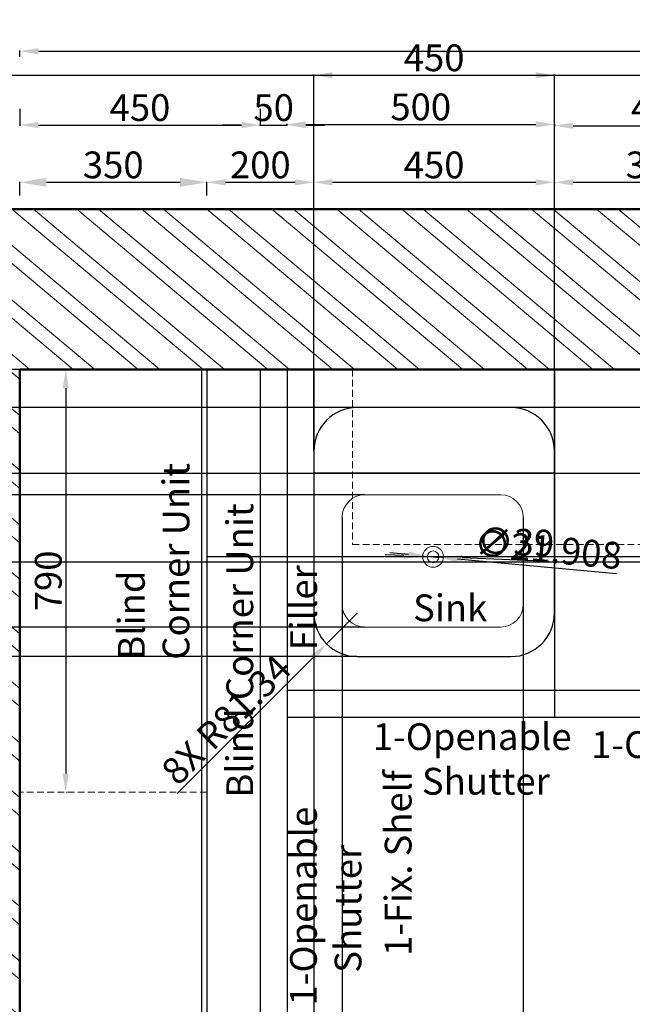
# Model space of a CAD drawing. Units: millimetres. Extents: x 407065 to 421840, y 1168257 to 1177792.
# Tile 6 of 17: x 408024 to 409170, y 1175951 to 1177792. Entities that reach past the tile are written whole.
import ezdxf

# ---------------------------------------------------------------- set-up
doc = ezdxf.new("R2010")
doc.units = ezdxf.units.MM
doc.linetypes.add('DASHED', pattern=[19.05, 12.7, -6.35])
for name, color, linetype, lineweight in [('A-ANNO-DIMS', 6, 'Continuous', 18), ('A-ANNO-TEXT', 30, 'Continuous', 18), ('A-EQPM', 8, 'Continuous', 18), ('A-FURN', 3, 'Continuous', 25), ('A-FURN-HIDN', 7, 'DASHED', 18), ('A-WALL', 7, 'Continuous', 50), ('A-WALL-PATT', 8, 'Continuous', 13)]:
    doc.layers.add(name, color=color, linetype=linetype, lineweight=lineweight)
doc.styles.get("Standard").update_dxf_attribs({"font": 'arial.ttf'})
doc.dimstyles.new('ISO-25', dxfattribs={"dimtxt": 50, "dimasz": 35, "dimexe": 1.25, "dimexo": 0.625, "dimtad": 1, "dimdec": 1, "dimtxsty": 'Standard', "dimcen": 35, "dimadec": 0, "dimazin": 0, "dimtfac": 1, "dimtdec": 1, "dimtmove": 0, "dimatfit": 3, "dimfxl": 1, "dimarcsym": 0})

# ---------------------------------------------------------------- blocks, each defined once
blk = doc.blocks.new('*D1')
at = {"layer": 'A-ANNO-DIMS', "color": 0, "lineweight": -2, "transparency": 16777216}
for p, q in [((408024.3, 1177462.8), (408024.3, 1177488.9)), ((408074.3, 1177487.7), (408324.3, 1177487.7)), ((408374.3, 1177462.8), (408374.3, 1177488.9))]:
    blk.add_line(p, q, dxfattribs=at)
at = {"layer": 'A-ANNO-DIMS', "color": 0, "transparency": 16777216}
for points in [[(408074.3, 1177496), (408074.3, 1177479.3), (408024.3, 1177487.7)], [(408324.3, 1177496), (408324.3, 1177479.3), (408374.3, 1177487.7)]]:
    blk.add_solid(points, dxfattribs=at)
at = {"layer": 'Defpoints', "color": 0, "transparency": 16777216}
for p in [(408374.3, 1177487.7), (408024.3, 1177462.1), (408374.3, 1177462.1)]:
    blk.add_point(p, dxfattribs=at)
at = {"layer": 'A-ANNO-DIMS', "color": 0, "transparency": 16777216, "insert": (408199.3, 1177513.8), "char_height": 50, "attachment_point": 5}
blk.add_mtext('350', dxfattribs=at)
blk = doc.blocks.new('*D2')
at = {"layer": 'A-ANNO-DIMS', "color": 0, "lineweight": -2, "transparency": 16777216}
for p, q in [((408374.3, 1177462.8), (408374.3, 1177488.9)), ((408409.3, 1177487.7), (408539.3, 1177487.7)), ((408574.3, 1177462.8), (408574.3, 1177488.9))]:
    blk.add_line(p, q, dxfattribs=at)
at = {"layer": 'A-ANNO-DIMS', "color": 0, "transparency": 16777216}
for points in [[(408409.3, 1177493.5), (408409.3, 1177481.8), (408374.3, 1177487.7)], [(408539.3, 1177493.5), (408539.3, 1177481.8), (408574.3, 1177487.7)]]:
    blk.add_solid(points, dxfattribs=at)
at = {"layer": 'Defpoints', "color": 0, "transparency": 16777216}
for p in [(408574.3, 1177487.7), (408374.3, 1177462.1), (408574.3, 1177462.1)]:
    blk.add_point(p, dxfattribs=at)
at = {"layer": 'A-ANNO-DIMS', "color": 0, "transparency": 16777216, "insert": (408474.3, 1177513.8), "char_height": 50, "attachment_point": 5}
blk.add_mtext('200', dxfattribs=at)
blk = doc.blocks.new('*D3')
at = {"layer": 'A-ANNO-DIMS', "color": 0, "lineweight": -2, "transparency": 16777216}
for p, q in [((408574.3, 1177488.3), (408574.3, 1177488.9)), ((408609.3, 1177487.7), (408989.3, 1177487.7)), ((409024.3, 1177487), (409024.3, 1177486.4))]:
    blk.add_line(p, q, dxfattribs=at)
at = {"layer": 'A-ANNO-DIMS', "color": 0, "transparency": 16777216}
for points in [[(408609.3, 1177493.5), (408609.3, 1177481.8), (408574.3, 1177487.7)], [(408989.3, 1177493.5), (408989.3, 1177481.8), (409024.3, 1177487.7)]]:
    blk.add_solid(points, dxfattribs=at)
at = {"layer": 'Defpoints', "color": 0, "transparency": 16777216}
for p in [(408574.3, 1177487.7), (409024.3, 1177487.7), (409024.3, 1177487.7)]:
    blk.add_point(p, dxfattribs=at)
at = {"layer": 'A-ANNO-DIMS', "color": 0, "transparency": 16777216, "insert": (408799.3, 1177513.8), "char_height": 50, "attachment_point": 5}
blk.add_mtext('450', dxfattribs=at)
blk = doc.blocks.new('*D4')
at = {"layer": 'A-ANNO-DIMS', "color": 0, "lineweight": -2, "transparency": 16777216}
for p, q in [((409024.3, 1177488.3), (409024.3, 1177488.9)), ((409059.3, 1177487.7), (409369.3, 1177487.7)), ((409404.3, 1177488.3), (409404.3, 1177488.9))]:
    blk.add_line(p, q, dxfattribs=at)
at = {"layer": 'A-ANNO-DIMS', "color": 0, "transparency": 16777216}
for points in [[(409059.3, 1177493.5), (409059.3, 1177481.8), (409024.3, 1177487.7)], [(409369.3, 1177493.5), (409369.3, 1177481.8), (409404.3, 1177487.7)]]:
    blk.add_solid(points, dxfattribs=at)
at = {"layer": 'Defpoints', "color": 0, "transparency": 16777216}
for p in [(409024.3, 1177487.7), (409404.3, 1177487.7), (409404.3, 1177487.7)]:
    blk.add_point(p, dxfattribs=at)
at = {"layer": 'A-ANNO-DIMS', "color": 0, "transparency": 16777216, "insert": (409214.3, 1177513.8), "char_height": 50, "attachment_point": 5}
blk.add_mtext('380', dxfattribs=at)
blk = doc.blocks.new('*D8')
at = {"layer": 'A-ANNO-DIMS', "color": 0, "lineweight": -2, "transparency": 16777216}
for p, q in [((408024.3, 1177625.1), (408024.3, 1177593.5)), ((408474.3, 1177625.1), (408474.3, 1177593.5)), ((408059.3, 1177594.8), (408439.3, 1177594.8))]:
    blk.add_line(p, q, dxfattribs=at)
at = {"layer": 'A-ANNO-DIMS', "color": 0, "transparency": 16777216}
for points in [[(408059.3, 1177600.6), (408059.3, 1177588.9), (408024.3, 1177594.8)], [(408439.3, 1177600.6), (408439.3, 1177588.9), (408474.3, 1177594.8)]]:
    blk.add_solid(points, dxfattribs=at)
at = {"layer": 'Defpoints', "color": 0, "transparency": 16777216}
for p in [(408024.3, 1177625.8), (408474.3, 1177625.8), (408474.3, 1177594.8)]:
    blk.add_point(p, dxfattribs=at)
at = {"layer": 'A-ANNO-DIMS', "color": 0, "transparency": 16777216, "insert": (408249.3, 1177620.9), "char_height": 50, "attachment_point": 5}
blk.add_mtext('450', dxfattribs=at)
blk = doc.blocks.new('*D9')
at = {"layer": 'A-ANNO-DIMS', "color": 0, "lineweight": -2, "transparency": 16777216}
for p, q in [((408439.3, 1177594.8), (408404.3, 1177594.8)), ((408474.3, 1177594.1), (408474.3, 1177596)), ((408474.3, 1177594.8), (408524.3, 1177594.8)), ((408524.3, 1177594.1), (408524.3, 1177596)), ((408559.3, 1177594.8), (408594.3, 1177594.8))]:
    blk.add_line(p, q, dxfattribs=at)
at = {"layer": 'A-ANNO-DIMS', "color": 0, "transparency": 16777216}
for points in [[(408439.3, 1177600.6), (408439.3, 1177588.9), (408474.3, 1177594.8)], [(408559.3, 1177600.6), (408559.3, 1177588.9), (408524.3, 1177594.8)]]:
    blk.add_solid(points, dxfattribs=at)
at = {"layer": 'Defpoints', "color": 0, "transparency": 16777216}
for p in [(408474.3, 1177593.5), (408524.3, 1177594.8), (408524.3, 1177593.5)]:
    blk.add_point(p, dxfattribs=at)
at = {"layer": 'A-ANNO-DIMS', "color": 0, "transparency": 16777216, "insert": (408499.3, 1177620.9), "char_height": 50, "attachment_point": 5}
blk.add_mtext('50', dxfattribs=at)
blk = doc.blocks.new('*D10')
at = {"layer": 'A-ANNO-DIMS', "color": 0, "lineweight": -2, "transparency": 16777216}
for p, q in [((408524.3, 1177594.1), (408524.3, 1177597.3)), ((408559.3, 1177596), (408989.3, 1177596)), ((409024.3, 1177594.1), (409024.3, 1177597.3))]:
    blk.add_line(p, q, dxfattribs=at)
at = {"layer": 'A-ANNO-DIMS', "color": 0, "transparency": 16777216}
for points in [[(408559.3, 1177601.8), (408559.3, 1177590.2), (408524.3, 1177596)], [(408989.3, 1177601.8), (408989.3, 1177590.2), (409024.3, 1177596)]]:
    blk.add_solid(points, dxfattribs=at)
at = {"layer": 'Defpoints', "color": 0, "transparency": 16777216}
for p in [(408524.3, 1177593.5), (409024.3, 1177596), (409024.3, 1177593.5)]:
    blk.add_point(p, dxfattribs=at)
at = {"layer": 'A-ANNO-DIMS', "color": 0, "transparency": 16777216, "insert": (408774.3, 1177622.2), "char_height": 50, "attachment_point": 5}
blk.add_mtext('500', dxfattribs=at)
blk = doc.blocks.new('*D11')
at = {"layer": 'A-ANNO-DIMS', "color": 0, "lineweight": -2, "transparency": 16777216}
for p, q in [((409024.3, 1177596.6), (409024.3, 1177592.3)), ((409059.3, 1177593.5), (409389.3, 1177593.5)), ((409424.3, 1177596.6), (409424.3, 1177592.3))]:
    blk.add_line(p, q, dxfattribs=at)
at = {"layer": 'A-ANNO-DIMS', "color": 0, "transparency": 16777216}
for points in [[(409059.3, 1177599.3), (409059.3, 1177587.7), (409024.3, 1177593.5)], [(409389.3, 1177599.3), (409389.3, 1177587.7), (409424.3, 1177593.5)]]:
    blk.add_solid(points, dxfattribs=at)
at = {"layer": 'Defpoints', "color": 0, "transparency": 16777216}
for p in [(409024.3, 1177597.3), (409424.3, 1177597.3), (409424.3, 1177593.5)]:
    blk.add_point(p, dxfattribs=at)
at = {"layer": 'A-ANNO-DIMS', "color": 0, "transparency": 16777216, "insert": (409224.3, 1177619.7), "char_height": 50, "attachment_point": 5}
blk.add_mtext('400', dxfattribs=at)
blk = doc.blocks.new('*D16')
at = {"layer": 'A-ANNO-DIMS', "color": 0, "lineweight": -2, "transparency": 16777216}
for p, q in [((408024.3, 1177722.1), (408024.3, 1177733.9)), ((408059.3, 1177732.7), (410789.3, 1177732.7)), ((410824.3, 1177722.1), (410824.3, 1177733.9))]:
    blk.add_line(p, q, dxfattribs=at)
at = {"layer": 'A-ANNO-DIMS', "color": 0, "transparency": 16777216}
for points in [[(408059.3, 1177738.5), (408059.3, 1177726.8), (408024.3, 1177732.7)], [(410789.3, 1177738.5), (410789.3, 1177726.8), (410824.3, 1177732.7)]]:
    blk.add_solid(points, dxfattribs=at)
at = {"layer": 'Defpoints', "color": 0, "transparency": 16777216}
for p in [(410824.3, 1177732.7), (408024.3, 1177721.4), (410824.3, 1177721.4)]:
    blk.add_point(p, dxfattribs=at)
at = {"layer": 'A-ANNO-DIMS', "color": 0, "transparency": 16777216, "insert": (409424.3, 1177758.8), "char_height": 50, "attachment_point": 5}
blk.add_mtext('2800', dxfattribs=at)
blk = doc.blocks.new('*D36')
at = {"layer": 'A-ANNO-DIMS', "color": 0, "lineweight": -2, "transparency": 16777216}
for p, q in [((408111.1, 1177137.8), (408111.7, 1177137.8)), ((408110.5, 1177102.8), (408110.5, 1176382.8)), ((408111.1, 1176347.8), (408111.7, 1176347.8))]:
    blk.add_line(p, q, dxfattribs=at)
at = {"layer": 'A-ANNO-DIMS', "color": 0, "transparency": 16777216}
for points in [[(408104.6, 1177102.8), (408116.3, 1177102.8), (408110.5, 1177137.8)], [(408104.6, 1176382.8), (408116.3, 1176382.8), (408110.5, 1176347.8)]]:
    blk.add_solid(points, dxfattribs=at)
at = {"layer": 'Defpoints', "color": 0, "transparency": 16777216}
for p in [(408110.5, 1177137.8), (408110.5, 1176347.8), (408110.5, 1176347.8)]:
    blk.add_point(p, dxfattribs=at)
at = {"layer": 'A-ANNO-DIMS', "color": 0, "transparency": 16777216, "insert": (408084.3, 1176742.8), "char_height": 50, "attachment_point": 5, "rotation": 90}
blk.add_mtext('790', dxfattribs=at)
blk = doc.blocks.new('*D165')
at = {"layer": 'A-ANNO-DIMS', "color": 0, "lineweight": -2, "transparency": 16777216}
for p, q in [((407724.3, 1177438.4), (407724.3, 1177689)), ((407759.3, 1177687.8), (410989.3, 1177687.8)), ((411024.3, 1177438.4), (411024.3, 1177689))]:
    blk.add_line(p, q, dxfattribs=at)
at = {"layer": 'A-ANNO-DIMS', "color": 0, "transparency": 16777216}
for points in [[(407759.3, 1177693.6), (407759.3, 1177682), (407724.3, 1177687.8)], [(410989.3, 1177693.6), (410989.3, 1177682), (411024.3, 1177687.8)]]:
    blk.add_solid(points, dxfattribs=at)
at = {"layer": 'Defpoints', "color": 0, "transparency": 16777216}
for p in [(411024.3, 1177687.8), (407724.3, 1177437.8), (411024.3, 1177437.8)]:
    blk.add_point(p, dxfattribs=at)
at = {"layer": 'A-ANNO-DIMS', "color": 0, "transparency": 16777216, "insert": (409374.3, 1177714), "char_height": 50, "attachment_point": 5}
blk.add_mtext('3300', dxfattribs=at)
blk = doc.blocks.new('*D171')
at = {"layer": 'A-ANNO-DIMS', "color": 0, "lineweight": -2, "transparency": 16777216}
for p, q in [((408574.3, 1176986.1), (408574.3, 1177689)), ((408609.3, 1177687.8), (408989.3, 1177687.8)), ((409024.3, 1176986.1), (409024.3, 1177689))]:
    blk.add_line(p, q, dxfattribs=at)
at = {"layer": 'A-ANNO-DIMS', "color": 0, "transparency": 16777216}
for points in [[(408609.3, 1177693.6), (408609.3, 1177682), (408574.3, 1177687.8)], [(408989.3, 1177693.6), (408989.3, 1177682), (409024.3, 1177687.8)]]:
    blk.add_solid(points, dxfattribs=at)
at = {"layer": 'Defpoints', "color": 0, "transparency": 16777216}
for p in [(409024.3, 1177687.8), (408574.3, 1176985.5), (409024.3, 1176985.5)]:
    blk.add_point(p, dxfattribs=at)
at = {"layer": 'A-ANNO-DIMS', "color": 0, "transparency": 16777216, "insert": (408799.3, 1177713.9), "char_height": 50, "attachment_point": 5}
blk.add_mtext('450', dxfattribs=at)
blk = doc.blocks.new('*D172')
at = {"layer": 'A-ANNO-DIMS', "color": 0, "lineweight": -2, "transparency": 16777216}
for p, q in [((408655, 1177066.8), (407473.1, 1177066.8)), ((407474.3, 1177031.8), (407474.3, 1176636.4)), ((408655, 1176601.4), (407473.1, 1176601.4))]:
    blk.add_line(p, q, dxfattribs=at)
at = {"layer": 'A-ANNO-DIMS', "color": 0, "transparency": 16777216}
for points in [[(407468.5, 1177031.8), (407480.1, 1177031.8), (407474.3, 1177066.8)], [(407468.5, 1176636.4), (407480.1, 1176636.4), (407474.3, 1176601.4)]]:
    blk.add_solid(points, dxfattribs=at)
at = {"layer": 'Defpoints', "color": 0, "transparency": 16777216}
for p in [(408655.7, 1177066.8), (407474.3, 1176601.4), (408655.7, 1176601.4)]:
    blk.add_point(p, dxfattribs=at)
at = {"layer": 'A-ANNO-DIMS', "color": 0, "transparency": 16777216, "insert": (407448.2, 1176834.1), "char_height": 50, "attachment_point": 5, "rotation": 90}
blk.add_mtext('465.4', dxfattribs=at)
blk = doc.blocks.new('*D173')
at = {"layer": 'A-ANNO-DIMS', "color": 0, "lineweight": -2, "transparency": 16777216}
for p, q in [((407474.3, 1177172.8), (407474.3, 1177207.8)), ((408573.7, 1177137.8), (407473.1, 1177137.8)), ((407474.3, 1177137.8), (407474.3, 1177066.8)), ((408655, 1177066.8), (407473.1, 1177066.8)), ((407474.3, 1177031.8), (407474.3, 1176827.1))]:
    blk.add_line(p, q, dxfattribs=at)
at = {"layer": 'A-ANNO-DIMS', "color": 0, "transparency": 16777216}
for points in [[(407468.5, 1177172.8), (407480.1, 1177172.8), (407474.3, 1177137.8)], [(407468.5, 1177031.8), (407480.1, 1177031.8), (407474.3, 1177066.8)]]:
    blk.add_solid(points, dxfattribs=at)
at = {"layer": 'Defpoints', "color": 0, "transparency": 16777216}
for p in [(408574.3, 1177137.8), (407474.3, 1177066.8), (408655.7, 1177066.8)]:
    blk.add_point(p, dxfattribs=at)
at = {"layer": 'A-ANNO-DIMS', "color": 0, "transparency": 16777216, "insert": (407448.2, 1176912), "char_height": 50, "attachment_point": 5, "rotation": 90}
blk.add_mtext('70.98', dxfattribs=at)
blk = doc.blocks.new('*D174')
at = {"layer": 'A-ANNO-DIMS', "color": 0, "lineweight": -2, "transparency": 16777216}
for p, q in [((408627.4, 1176861), (408627.4, 1172896.5)), ((408966, 1176861), (408966, 1172896.5)), ((408662.4, 1172897.8), (408931, 1172897.8))]:
    blk.add_line(p, q, dxfattribs=at)
at = {"layer": 'A-ANNO-DIMS', "color": 0, "transparency": 16777216}
for points in [[(408662.4, 1172903.6), (408662.4, 1172892), (408627.4, 1172897.8)], [(408931, 1172903.6), (408931, 1172892), (408966, 1172897.8)]]:
    blk.add_solid(points, dxfattribs=at)
at = {"layer": 'Defpoints', "color": 0, "transparency": 16777216}
for p in [(408627.4, 1176861.7), (408966, 1176861.7), (408966, 1172897.8)]:
    blk.add_point(p, dxfattribs=at)
at = {"layer": 'A-ANNO-DIMS', "color": 0, "transparency": 16777216, "insert": (408796.7, 1172924), "char_height": 50, "attachment_point": 5}
blk.add_mtext('338.63', dxfattribs=at)
blk = doc.blocks.new('*D175')
at = {"layer": 'A-ANNO-DIMS', "color": 0, "lineweight": -2, "transparency": 16777216}
for p, q in [((408668.9, 1176903.8), (407473.1, 1176903.8)), ((407474.3, 1176868.8), (407474.3, 1176691.5)), ((408668.9, 1176656.5), (407473.1, 1176656.5))]:
    blk.add_line(p, q, dxfattribs=at)
at = {"layer": 'A-ANNO-DIMS', "color": 0, "transparency": 16777216}
for points in [[(407468.5, 1176868.8), (407480.1, 1176868.8), (407474.3, 1176903.8)], [(407468.5, 1176691.5), (407480.1, 1176691.5), (407474.3, 1176656.5)]]:
    blk.add_solid(points, dxfattribs=at)
at = {"layer": 'Defpoints', "color": 0, "transparency": 16777216}
for p in [(408669.5, 1176903.8), (407474.3, 1176656.5), (408669.5, 1176656.5)]:
    blk.add_point(p, dxfattribs=at)
at = {"layer": 'A-ANNO-DIMS', "color": 0, "transparency": 16777216, "insert": (407448.1, 1176780.2), "char_height": 50, "attachment_point": 5, "rotation": 90}
blk.add_mtext('247.3', dxfattribs=at)
blk = doc.blocks.new('*D176')
at = {"layer": 'A-ANNO-DIMS', "color": 0, "lineweight": -2, "transparency": 16777216}
for p, q in [((408574.3, 1176984.8), (408574.3, 1172896.5)), ((408627.4, 1176861), (408627.4, 1172896.5)), ((408539.3, 1172897.8), (408504.3, 1172897.8)), ((408574.3, 1172897.8), (408627.4, 1172897.8)), ((408662.4, 1172897.8), (408867.1, 1172897.8))]:
    blk.add_line(p, q, dxfattribs=at)
at = {"layer": 'A-ANNO-DIMS', "color": 0, "transparency": 16777216}
for points in [[(408539.3, 1172903.6), (408539.3, 1172892), (408574.3, 1172897.8)], [(408662.4, 1172903.6), (408662.4, 1172892), (408627.4, 1172897.8)]]:
    blk.add_solid(points, dxfattribs=at)
at = {"layer": 'Defpoints', "color": 0, "transparency": 16777216}
for p in [(408574.3, 1176985.5), (408627.4, 1176861.7), (408627.4, 1172897.8)]:
    blk.add_point(p, dxfattribs=at)
at = {"layer": 'A-ANNO-DIMS', "color": 0, "transparency": 16777216, "insert": (408782.2, 1172924), "char_height": 50, "attachment_point": 5}
blk.add_mtext('53.04', dxfattribs=at)
blk = doc.blocks.new('*D177')
at = {"layer": 'A-ANNO-DIMS', "color": 0, "lineweight": -2, "transparency": 16777216}
for p, q in [((408655, 1177066.8), (407473.1, 1177066.8)), ((407474.3, 1177031.8), (407474.3, 1176938.8)), ((408668.9, 1176903.8), (407473.1, 1176903.8))]:
    blk.add_line(p, q, dxfattribs=at)
at = {"layer": 'A-ANNO-DIMS', "color": 0, "transparency": 16777216}
for points in [[(407468.5, 1177031.8), (407480.1, 1177031.8), (407474.3, 1177066.8)], [(407468.5, 1176938.8), (407480.1, 1176938.8), (407474.3, 1176903.8)]]:
    blk.add_solid(points, dxfattribs=at)
at = {"layer": 'Defpoints', "color": 0, "transparency": 16777216}
for p in [(408655.7, 1177066.8), (407474.3, 1176903.8), (408669.5, 1176903.8)]:
    blk.add_point(p, dxfattribs=at)
at = {"layer": 'A-ANNO-DIMS', "color": 0, "transparency": 16777216, "insert": (407448.1, 1176985.3), "char_height": 50, "attachment_point": 5, "rotation": 90}
blk.add_mtext('163', dxfattribs=at)
blk = doc.blocks.new('*D182')
at = {"layer": 'A-ANNO-DIMS', "color": 0, "lineweight": -2, "transparency": 16777216}
for p, q in [((409505, 1177066.8), (407473.1, 1177066.8)), ((407474.3, 1177031.8), (407474.3, 1176978.3)), ((409523.4, 1176943.3), (407473.1, 1176943.3)), ((407474.3, 1176943.3), (407474.3, 1176742.7))]:
    blk.add_line(p, q, dxfattribs=at)
at = {"layer": 'A-ANNO-DIMS', "color": 0, "transparency": 16777216}
for points in [[(407468.5, 1177031.8), (407480.1, 1177031.8), (407474.3, 1177066.8)], [(407468.5, 1176978.3), (407480.1, 1176978.3), (407474.3, 1176943.3)]]:
    blk.add_solid(points, dxfattribs=at)
at = {"layer": 'Defpoints', "color": 0, "transparency": 16777216}
for p in [(409505.7, 1177066.8), (407474.3, 1176943.3), (409524, 1176943.3)]:
    blk.add_point(p, dxfattribs=at)
at = {"layer": 'A-ANNO-DIMS', "color": 0, "transparency": 16777216, "insert": (407448.1, 1176825.5), "char_height": 50, "attachment_point": 5, "rotation": 90}
blk.add_mtext('123.5', dxfattribs=at)
blk = doc.blocks.new('*D183')
at = {"layer": 'A-ANNO-DIMS', "color": 0, "lineweight": -2, "transparency": 16777216}
for p, q in [((409523.4, 1176943.3), (407473.1, 1176943.3)), ((407474.3, 1176908.3), (407474.3, 1176812.5)), ((409523.4, 1176777.5), (407473.1, 1176777.5)), ((407474.3, 1176777.5), (407474.3, 1176538.4))]:
    blk.add_line(p, q, dxfattribs=at)
at = {"layer": 'A-ANNO-DIMS', "color": 0, "transparency": 16777216}
for points in [[(407468.5, 1176908.3), (407480.1, 1176908.3), (407474.3, 1176943.3)], [(407468.5, 1176812.5), (407480.1, 1176812.5), (407474.3, 1176777.5)]]:
    blk.add_solid(points, dxfattribs=at)
at = {"layer": 'Defpoints', "color": 0, "transparency": 16777216}
for p in [(409524, 1176943.3), (407474.3, 1176777.5), (409524, 1176777.5)]:
    blk.add_point(p, dxfattribs=at)
at = {"layer": 'A-ANNO-DIMS', "color": 0, "transparency": 16777216, "insert": (407448.2, 1176640.4), "char_height": 50, "attachment_point": 5, "rotation": 90}
blk.add_mtext('165.86', dxfattribs=at)
blk = doc.blocks.new('*D223')
at = {"layer": 'A-ANNO-DIMS', "color": 0, "lineweight": -2, "transparency": 16777216}
for p, q in [((408655.7, 1176682.7), (408598.2, 1176625.2)), ((408319, 1176345.6), (408573.5, 1176600.4))]:
    blk.add_line(p, q, dxfattribs=at)
at = {"layer": 'A-ANNO-DIMS', "color": 0, "transparency": 16777216}
blk.add_solid([(408569.3, 1176604.5), (408577.6, 1176596.3), (408598.2, 1176625.2)], dxfattribs=at)
at = {"layer": 'Defpoints', "color": 0, "transparency": 16777216}
for p in [(408655.7, 1176682.7), (408598.2, 1176625.2)]:
    blk.add_point(p, dxfattribs=at)
at = {"layer": 'A-ANNO-DIMS', "color": 0, "transparency": 16777216, "insert": (408415.3, 1176479.1), "char_height": 50, "attachment_point": 5, "rotation": 45.0461}
blk.add_mtext('8X R81.34', dxfattribs=at)
blk = doc.blocks.new('*D229')
at = {"layer": 'A-ANNO-DIMS', "color": 0, "lineweight": -2, "transparency": 16777216}
for p, q in [((408743, 1176790), (408708, 1176791.4)), ((408777.9, 1176788.6), (408816.9, 1176787)), ((409014.1, 1176779), (408851.9, 1176785.6))]:
    blk.add_line(p, q, dxfattribs=at)
at = {"layer": 'A-ANNO-DIMS', "color": 0, "transparency": 16777216}
for points in [[(408743.2, 1176795.8), (408742.7, 1176784.2), (408777.9, 1176788.6)], [(408852.1, 1176791.4), (408851.7, 1176779.8), (408816.9, 1176787)]]:
    blk.add_solid(points, dxfattribs=at)
at = {"layer": 'Defpoints', "color": 0, "transparency": 16777216}
for p in [(408777.9, 1176788.6), (408816.9, 1176787)]:
    blk.add_point(p, dxfattribs=at)
at = {"layer": 'A-ANNO-DIMS', "color": 0, "transparency": 16777216, "insert": (408951.6, 1176809.1), "char_height": 50, "attachment_point": 5, "rotation": 357.6726}
blk.add_mtext('∅39', dxfattribs=at)
blk = doc.blocks.new('*D230')
at = {"layer": 'A-ANNO-DIMS', "color": 0, "lineweight": -2, "transparency": 16777216}
for p, q in [((408751.7, 1176792), (408716.8, 1176795.3)), ((408786.5, 1176788.8), (408808.3, 1176786.8)), ((409140.2, 1176756), (408843.2, 1176783.5))]:
    blk.add_line(p, q, dxfattribs=at)
at = {"layer": 'A-ANNO-DIMS', "color": 0, "transparency": 16777216}
for points in [[(408752.2, 1176797.9), (408751.1, 1176786.2), (408786.5, 1176788.8)], [(408843.7, 1176789.4), (408842.7, 1176777.7), (408808.3, 1176786.8)]]:
    blk.add_solid(points, dxfattribs=at)
at = {"layer": 'Defpoints', "color": 0, "transparency": 16777216}
for p in [(408786.5, 1176788.8), (408808.3, 1176786.8)]:
    blk.add_point(p, dxfattribs=at)
at = {"layer": 'A-ANNO-DIMS', "color": 0, "transparency": 16777216, "insert": (409011.7, 1176795.6), "char_height": 50, "attachment_point": 5, "rotation": 354.6966}
blk.add_mtext('∅21.908', dxfattribs=at)

msp = doc.modelspace()

# ---------------------------------------------------------------- hatches: boundary and pattern name
at = {"layer": 'A-WALL-PATT'}
h = msp.add_hatch(dxfattribs=at)
h.set_pattern_fill('ANSI32', color=256, scale=8.2, angle=95)
h.paths.add_polyline_path([(411024.3133, 1177437.7952), (407724.3133, 1177437.7952), (407724.3133, 1177137.7952), (408024.3133, 1177137.7952), (410824.3133, 1177137.7952), (411024.3133, 1177137.7952)])
h = msp.add_hatch(dxfattribs=at)
h.set_pattern_fill('ANSI32', color=256, scale=8.2, angle=95)
h.paths.add_polyline_path([(408024.3133, 1177137.7952), (407724.3133, 1177137.7952), (407724.3133, 1174467.7952), (408024.3133, 1174467.7952)])

# ---------------------------------------------------------------- linework, layer by layer
at = {"layer": 'A-EQPM'}
for p, q in [((408669.5202, 1176903.8236), (408923.8256, 1176903.8236)), ((408627.3554, 1176698.673), (408627.3554, 1176861.6588)), ((408965.9904, 1176861.6588), (408965.9904, 1176698.673)), ((408923.8256, 1176656.5082), (408669.5202, 1176656.5082))]:
    msp.add_line(p, q, dxfattribs=at)
for radius in [19.5001, 10.9538]:
    msp.add_circle((408797.4331, 1176787.7952), radius, dxfattribs=at)
for centre, start, end in [((408669.5202, 1176861.6588), 90, 180), ((408923.8256, 1176861.6588), 0, 90), ((408669.5202, 1176698.673), 180, 270), ((408923.8256, 1176698.673), 270, 0)]:
    msp.add_arc(centre, 42.1648, start, end, dxfattribs=at)
at = {"layer": 'A-FURN'}
for p, q in [((408364.3133, 1177137.7952), (408364.3133, 1174737.7952)), ((408374.3133, 1177137.7952), (408374.3133, 1174737.7952)), ((408474.3133, 1177137.7952), (408474.3133, 1174737.7952)), ((408524.3133, 1177137.7952), (408524.3133, 1174737.7952)), ((408574.3133, 1177137.7952), (408574.3133, 1176487.7952)), ((409024.3133, 1177137.7952), (409024.3133, 1176487.7952)), ((408574.3133, 1176944.8035), (409024.3133, 1176944.8035)), ((410474.3133, 1176787.7952), (408374.3133, 1176787.7952)), ((410224.3133, 1176537.7952), (408524.3133, 1176537.7952)), ((410224.3133, 1176487.7952), (408524.3133, 1176487.7952))]:
    msp.add_line(p, q, dxfattribs=at)
msp.add_lwpolyline([(408574.3133, 1176985.4747), (408574.3133, 1176682.7483, 0.414213562), (408655.6554, 1176601.4062), (408942.9713, 1176601.4062, 0.414213562), (409024.3133, 1176682.7483), (409024.3133, 1176985.4747, 0.414213562), (408942.9713, 1177066.8168), (408655.6554, 1177066.8168, 0.414213562)], format="xyb", close=True, dxfattribs=at)
at = {"layer": 'A-FURN-HIDN'}
for p, q in [((408646.6902, 1177137.7952), (408646.6902, 1176811.0192)), ((408646.6902, 1176811.0192), (409404.3149, 1176811.0044)), ((408374.3133, 1176347.7952), (408024.3133, 1176347.7952))]:
    msp.add_line(p, q, dxfattribs=at)
at = {"layer": 'A-WALL'}
for p, q in [((411024.3133, 1177437.7952), (407724.3133, 1177437.7952)), ((408024.3133, 1177137.7952), (408024.3133, 1174467.7952)), ((410824.3133, 1177137.7952), (408024.3133, 1177137.7952))]:
    msp.add_line(p, q, dxfattribs=at)

# ---------------------------------------------------------------- texts
at = {"layer": 'A-ANNO-TEXT', "char_height": 50, "attachment_point": 1, "rotation": 90}
for s, width, insert in [('Blind Corner Unit', 382.409863, (408208.2479, 1176595.3965)), ('Blind Corner Unit', 580.329145, (408410.8983, 1176337.8377)), ('     Filler', 382.409863, (408530.1747, 1176536.3452)), ('  1-Fix. Shelf', 382.409863, (408707.1122, 1176011.1357)), ('  1-Openable \\P      Shutter', 804.918817, (408530.0096, 1175918.7328))]:
    msp.add_mtext_dynamic_manual_height_columns(s, width=width, gutter_width=12.5, heights=[0], dxfattribs=dict(at, insert=insert))
at = {"layer": 'A-ANNO-TEXT', "char_height": 50, "attachment_point": 1}
for s, insert in [('Sink', (408760.003, 1176717.3734)), ('  1-Openable\\P      Shutter', (408684.8484, 1176476.6835)), ('  1-Openable\\P      Shutter', (409092.9692, 1176461.7378))]:
    msp.add_mtext_dynamic_manual_height_columns(s, width=382.409863, gutter_width=12.5, heights=[0], dxfattribs=dict(at, insert=insert))

# ---------------------------------------------------------------- dimensions: what is measured, and where the dimension line sits
at = {"layer": 'A-ANNO-DIMS'}
for base, p1, p2, override, picture, middle in [((410824.3133, 1177732.6671), (408024.3133, 1177721.4288), (410824.3133, 1177721.4288), {"dimclrd": 0, "dimclre": 0, "dimclrt": 0}, '*D16', (409424.3133, 1177758.8207)), ((411024.3133, 1177687.7952), (407724.3133, 1177437.7952), (411024.3133, 1177437.7952), {"dimdec": 0, "dimlfac": 1, "dimrnd": 0, "dimzin": 0, "dimdsep": 46, "dimlunit": 2}, '*D165', (409374.3133, 1177713.9659)), ((409024.3133, 1177687.7952), (408574.3133, 1176985.4747), (409024.3133, 1176985.4747), {"dimdec": 0, "dimlfac": 1, "dimrnd": 0, "dimzin": 0, "dimdsep": 46, "dimlunit": 2}, '*D171', (408799.3133, 1177713.9489)), ((408474.3133, 1177594.7623), (408024.3133, 1177625.7516), (408474.3133, 1177625.7516), {"dimclrd": 0, "dimclre": 0, "dimclrt": 0}, '*D8', (408249.3133, 1177620.916)), ((409024.3133, 1177596.0123), (408524.3133, 1177593.5123), (409024.3133, 1177593.5123), {"dimclrd": 0, "dimclre": 0, "dimclrt": 0}, '*D10', (408774.3133, 1177622.166)), ((409424.3133, 1177593.5123), (409024.3133, 1177597.2623), (409424.3133, 1177597.2623), {"dimclrd": 0, "dimclre": 0, "dimclrt": 0}, '*D11', (409224.3133, 1177619.666)), ((408374.3133, 1177487.6532), (408024.3133, 1177462.1391), (408374.3133, 1177462.1391), {"dimtxt": 50, "dimasz": 50, "dimclrd": 0, "dimclre": 0, "dimclrt": 0}, '*D1', (408199.3133, 1177513.8239)), ((408574.3133, 1177487.6532), (408374.3133, 1177462.1391), (408574.3133, 1177462.1391), {"dimclrd": 0, "dimclre": 0, "dimclrt": 0}, '*D2', (408474.3133, 1177513.8068)), ((409024.3133, 1177487.6532), (408574.3133, 1177487.6532), (409024.3133, 1177487.6532), {"dimclrd": 0, "dimclre": 0, "dimclrt": 0}, '*D3', (408799.3133, 1177513.8068)), ((409404.3149, 1177487.6532), (409024.3133, 1177487.6532), (409404.3149, 1177487.6532), {"dimclrd": 0, "dimclre": 0, "dimclrt": 0}, '*D4', (409214.3141, 1177513.8239)), ((408627.3554, 1172897.7952), (408574.3133, 1176985.4747), (408627.3554, 1176861.6588), {"dimdec": 2, "dimlfac": 1, "dimrnd": 0, "dimzin": 0, "dimdsep": 46, "dimlunit": 2}, '*D176', (408782.2403, 1172923.9659)), ((408965.99043, 1172897.79525), (408627.35545, 1176861.65877), (408965.99043, 1176861.65877), {"dimdec": 2, "dimlfac": 1, "dimrnd": 0, "dimzin": 0, "dimdsep": 46, "dimlunit": 2}, '*D174', (408796.67294, 1172923.96595))]:
    dim = msp.add_linear_dim(base=base, p1=p1, p2=p2, dimstyle='ISO-25', override=override, dxfattribs=at)
    dim.commit()
    dim.dimension.update_dxf_attribs({"geometry": picture, "text_midpoint": middle})
dim = msp.add_linear_dim(base=(408524.3133, 1177594.7623), p1=(408474.3133, 1177593.5123), p2=(408524.3133, 1177593.5123), dimstyle='ISO-25', override={"dimclrd": 0, "dimclre": 0, "dimclrt": 0}, dxfattribs=at)
dim.commit()
dim.dimension.update_dxf_attribs({"geometry": '*D9', "text_midpoint": (408499.3133, 1177594.7623), "dimtype": 160})
for base, p1, p2, override, picture, middle in [((407474.3133, 1177066.8168), (408574.3133, 1177137.7952), (408655.6554, 1177066.8168), {"dimdec": 2, "dimlfac": 1, "dimrnd": 0, "dimzin": 0, "dimdsep": 46, "dimlunit": 2}, '*D173', (407448.1597, 1176911.983)), ((408110.4821, 1176347.7952), (408110.4821, 1177137.7952), (408110.4821, 1176347.7952), {"dimclrd": 0, "dimclre": 0, "dimclrt": 0}, '*D36', (408084.3284, 1176742.7952)), ((407474.3133, 1176903.8236), (408655.6554, 1177066.8168), (408669.5202, 1176903.8236), {"dimdec": 0, "dimlfac": 1, "dimrnd": 0, "dimzin": 0, "dimdsep": 46, "dimlunit": 2}, '*D177', (407448.1426, 1176985.3202)), ((407474.3133, 1176943.3161), (409505.6554, 1177066.8168), (409524.0157, 1176943.3161), {"dimdec": 1, "dimlfac": 1, "dimrnd": 0, "dimzin": 0, "dimdsep": 46, "dimlunit": 2}, '*D182', (407448.1426, 1176825.4947)), ((407474.3133, 1176601.4062), (408655.6554, 1177066.8168), (408655.6554, 1176601.4062), {"dimdec": 1, "dimlfac": 1, "dimrnd": 0, "dimzin": 0, "dimdsep": 46, "dimlunit": 2}, '*D172', (407448.1597, 1176834.1115)), ((407474.3133, 1176777.4536), (409524.0157, 1176943.3161), (409524.0157, 1176777.4536), {"dimdec": 2, "dimlfac": 1, "dimrnd": 0, "dimzin": 0, "dimdsep": 46, "dimlunit": 2}, '*D183', (407448.1597, 1176640.4132)), ((407474.3133, 1176656.5082), (408669.5202, 1176903.8236), (408669.5202, 1176656.5082), {"dimdec": 1, "dimlfac": 1, "dimrnd": 0, "dimzin": 0, "dimdsep": 46, "dimlunit": 2}, '*D175', (407448.1426, 1176780.1659))]:
    dim = msp.add_linear_dim(base=base, p1=p1, p2=p2, angle=90, dimstyle='ISO-25', override=override, dxfattribs=at)
    dim.commit()
    dim.dimension.update_dxf_attribs({"geometry": picture, "text_midpoint": middle})
for p1, p2, override, picture, middle in [((408777.9491, 1176788.5871), (408816.9171, 1176787.0034), {"dimdec": 0, "dimlfac": 1, "dimrnd": 0, "dimzin": 0, "dimdsep": 46, "dimlunit": 2}, '*D229', (408950.4945, 1176781.5745)), ((408786.5262, 1176788.8077), (408808.34, 1176786.7828), {"dimdec": 3, "dimlfac": 1, "dimrnd": 0, "dimzin": 0, "dimdsep": 46, "dimlunit": 2}, '*D230', (409009.1386, 1176768.1431))]:
    dim = msp.add_diameter_dim_2p(p1=p1, p2=p2, dimstyle='ISO-25', override=override, dxfattribs=at)
    dim.commit()
    dim.dimension.update_dxf_attribs({"geometry": picture, "text_midpoint": middle})
dim = msp.add_radius_dim(center=(408655.6554, 1176682.7483), mpoint=(408598.1842, 1176625.1845), text='8X <>', dimstyle='ISO-25', override={"dimdec": 2, "dimlfac": 1, "dimrnd": 0, "dimzin": 0, "dimdsep": 46, "dimlunit": 2}, dxfattribs=at)
dim.commit()
dim.dimension.update_dxf_attribs({"geometry": '*D223', "text_midpoint": (408415.3498, 1176479.0964)})

doc.saveas('drawing.dxf')
